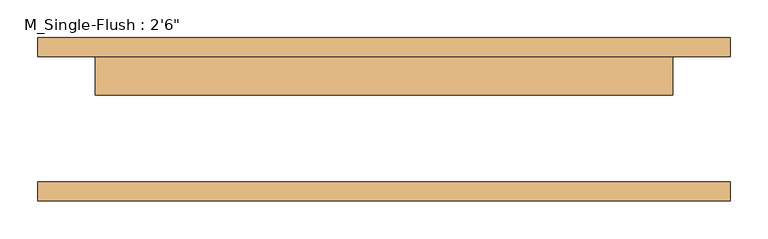
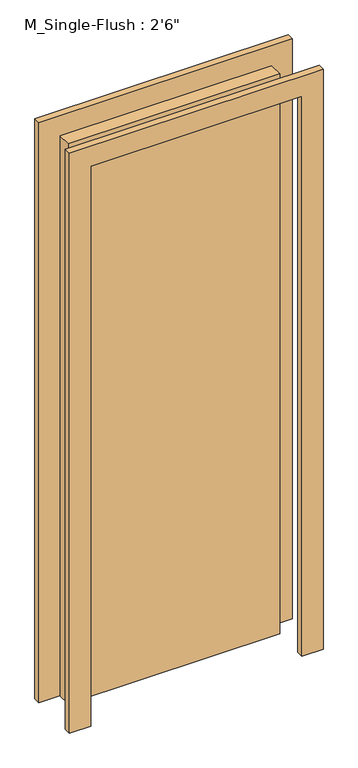
"""IFC4 building model written with IfcOpenShell, lengths in millimetres: door geometry."""

from ifc_helpers import new_model, si_unit, frame, origin, origin_with_axes, place, context, project, spatial, polyline, outline, extrude, source, transform, mapped, element, save


def door_e1312905(model_context):
    return source(origin(), model_context, "Body", "SweptSolid", [
        extrude(outline(polyline([(2209.6, -457.0), (0.0, -457.0), (0.0, -381.0), (2133.6, -381.0), (2133.6, 381.0), (0.0, 381.0), (0.0, 457.0), (2209.6, 457.0), (2209.6, -457.0)])), frame((0.0, 82.9, 0.0), z_axis=(0.0, 1.0, 0.0), x_axis=(0.0, 0.0, 1.0)), (0.0, 0.0, 1.0), 25.0),
        extrude(outline(polyline([(2209.6, 457.0), (2209.6, -457.0), (0.0, -457.0), (0.0, -381.0), (2133.6, -381.0), (2133.6, 381.0), (0.0, 381.0), (0.0, 457.0), (2209.6, 457.0)])), frame((0.0, -107.9, 0.0), z_axis=(0.0, 1.0, 0.0), x_axis=(0.0, 0.0, 1.0)), (0.0, 0.0, 1.0), 25.0),
        extrude(outline(polyline([(381.0, 31.9), (-381.0, 31.9), (-381.0, 82.9), (381.0, 82.9), (381.0, 31.9)])), origin_with_axes(), (0.0, 0.0, 1.0), 2133.6),
    ])


if __name__ == "__main__":
    model = new_model("IFC4")
    model_context = context("Model", 3, world=origin())
    ifc_project = project(units=[si_unit("LENGTHUNIT", "METRE", prefix="MILLI")], contexts=[model_context])
    site = spatial("IfcSite", under=ifc_project)
    building = spatial("IfcBuilding", under=site)
    placement = place(None, origin())
    door_shape = door_e1312905(model_context)
    element("IfcDoor", 1, ObjectType="M_Single-Flush : 2'6\"", at=placement, inside=building, context=model_context, shape_type="MappedRepresentation", body=[
        mapped(door_shape, transform((0.0, 0.0, 0.0), x_axis=(1.0, 0.0, 0.0), y_axis=(0.0, 1.0, 0.0), z_axis=(0.0, 0.0, 1.0))),
    ])
    save(model, "model.ifc")

# Revit data of these elements
# Type "M_Single-Flush : 2'6\""
#   Type Mark = "22"
#   Thickness = 0' - 2.00787"
#   Height = 7' - 0"
#   Trim Projection Ext = 0' - 0.98425"
#   Trim Projection Int = 0' - 0.98425"
#   Trim Width = 0' - 2.99213"
#   Width = 2' - 6"
#   Door Material = Door - Panel
#   Frame Material = Door - Frame
#   Function = (empty or 0)
#   Wall Closure = (empty or 0)
# Element 1 (IfcDoor, "M_Single-Flush : 2'6\"")
#   Materials on its faces: "Door - Frame", "Door - Panel"
# Materials
#   "Door - Panel": class "Wood", colour RGB 114 82 51, transparency 0
#   "Door - Frame": colour RGB 153 76 43, transparency 0
